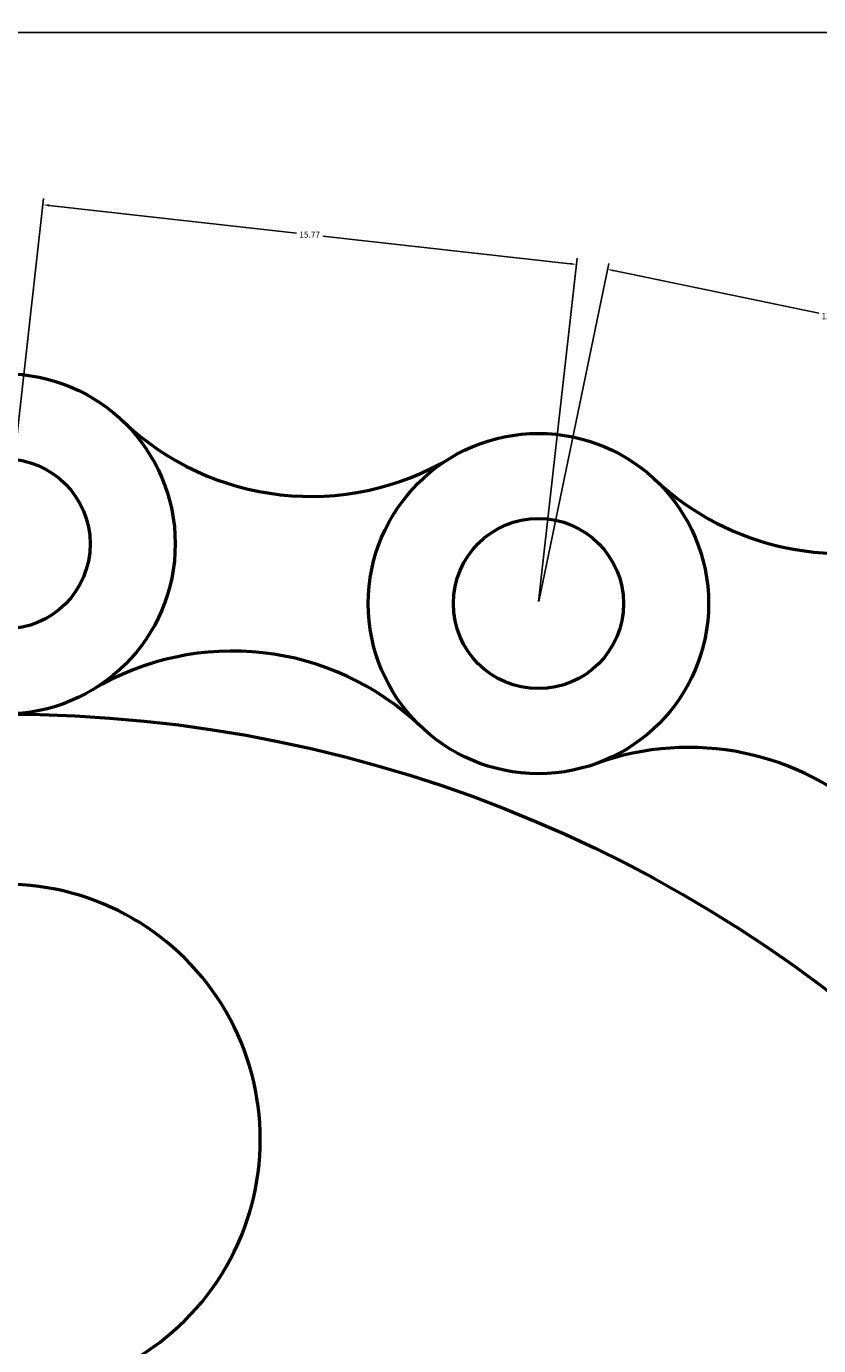
# Model space of a CAD drawing. Units: inches. Extents: x 413 to 622, y 326 to 447.
# Tile 7 of 15: x 473 to 497, y 408 to 447. Entities that reach past the tile are written whole.
import ezdxf

# ---------------------------------------------------------------- set-up
doc = ezdxf.new("R2010")
doc.units = ezdxf.units.IN
doc.header["$MEASUREMENT"] = 0
doc.layers.add('M-DIMS', color=2, linetype='Continuous', lineweight=18)
doc.layers.add('M-OUTL', color=7, linetype='Continuous', lineweight=50)
doc.styles.get("Standard").update_dxf_attribs({"font": 'arial.ttf'})
doc.dimstyles.get("Standard").update_dxf_attribs({"dimtxt": 0.18, "dimasz": 0.18, "dimexe": 0.18, "dimexo": 0.0625, "dimgap": 0.09, "dimtad": 0, "dimtih": 1, "dimtoh": 1, "dimdec": 4, "dimzin": 0, "dimdsep": 46, "dimtxsty": 'Standard', "dimcen": 0.09, "dimadec": 0, "dimazin": 0, "dimtfac": 1, "dimtdec": 4, "dimtofl": 0, "dimtmove": 0, "dimatfit": 3, "dimfxl": 1, "dimtolj": 1, "dimtzin": 0, "dimarcsym": 0})

# ---------------------------------------------------------------- blocks, each defined once
blk = doc.blocks.new('CHAIN-ROLLER-PIN')
for radius in [5, 2.5]:
    blk.add_circle((5, 5), radius)
blk = doc.blocks.new('SPROCKET-WEB-SLOT')
blk.add_arc((7.501, 21.25), 7.5, 30, 210)
blk = doc.blocks.new('CHAIN-LINK-WAIST-P15_769')
for centre, start, end in [((6.414, 14.762), 226.2787, 300.9551), ((4.115, -5.782), 46.2787, 120.9551)]:
    blk.add_arc(centre, 8, start, end)
blk = doc.blocks.new('CHAIN-LINK-WAIST-P13_603')
for centre, start, end in [((7.205, 15.87), 226.7719, 289.8627), ((2.718, -5.829), 46.7719, 109.8627)]:
    blk.add_arc(centre, 8, start, end)
blk = doc.blocks.new('*D11')
at = {"layer": 'Defpoints', "color": 0, "transparency": 16777216}
for p in [(621.66, 446.422), (621.66, 388.074), (423.314, 378.888)]:
    blk.add_point(p, dxfattribs=at)
at = {"layer": 'M-DIMS', "color": 0, "lineweight": -2, "transparency": 16777216}
for p, q in [((423.314, 378.95), (423.314, 446.602)), ((423.494, 446.422), (522.031, 446.422)), ((621.48, 446.422), (522.943, 446.422)), ((621.66, 388.137), (621.66, 446.602))]:
    blk.add_line(p, q, dxfattribs=at)
at = {"layer": 'M-DIMS', "color": 0, "transparency": 16777216}
for points in [[(423.494, 446.452), (423.494, 446.392), (423.314, 446.422)], [(621.48, 446.452), (621.48, 446.392), (621.66, 446.422)]]:
    blk.add_solid(points, dxfattribs=at)
at = {"layer": 'M-DIMS', "color": 0, "transparency": 16777216, "insert": (522.487, 446.422), "char_height": 0.18, "attachment_point": 5}
blk.add_mtext('\\A1;198.35', dxfattribs=at)
blk = doc.blocks.new('*D16')
at = {"layer": 'Defpoints', "color": 0, "transparency": 16777216}
for p in [(489.47, 439.607), (472.684, 431.392), (488.355, 429.638)]:
    blk.add_point(p, dxfattribs=at)
at = {"layer": 'M-DIMS', "color": 0, "lineweight": -2, "transparency": 16777216}
for p, q in [((472.691, 431.454), (473.819, 441.539)), ((473.978, 441.34), (481.249, 440.526)), ((489.292, 439.627), (482.02, 440.44)), ((488.362, 429.7), (489.49, 439.786))]:
    blk.add_line(p, q, dxfattribs=at)
at = {"layer": 'M-DIMS', "color": 0, "transparency": 16777216}
for points in [[(473.981, 441.37), (473.974, 441.31), (473.799, 441.36)], [(489.295, 439.656), (489.288, 439.597), (489.47, 439.607)]]:
    blk.add_solid(points, dxfattribs=at)
at = {"layer": 'M-DIMS', "color": 0, "transparency": 16777216, "insert": (481.635, 440.483), "char_height": 0.18, "attachment_point": 5}
blk.add_mtext('\\A1;15.77', dxfattribs=at)
blk = doc.blocks.new('*D17')
at = {"layer": 'Defpoints', "color": 0, "transparency": 16777216}
for p in [(503.707, 436.707), (488.355, 429.638), (501.676, 426.884)]:
    blk.add_point(p, dxfattribs=at)
at = {"layer": 'M-DIMS', "color": 0, "lineweight": -2, "transparency": 16777216}
for p, q in [((488.368, 429.7), (490.423, 439.637)), ((490.563, 439.425), (496.592, 438.178)), ((503.531, 436.743), (497.502, 437.99)), ((501.689, 426.945), (503.744, 436.883))]:
    blk.add_line(p, q, dxfattribs=at)
at = {"layer": 'M-DIMS', "color": 0, "transparency": 16777216}
for points in [[(490.569, 439.454), (490.557, 439.395), (490.386, 439.461)], [(503.537, 436.772), (503.525, 436.714), (503.707, 436.707)]]:
    blk.add_solid(points, dxfattribs=at)
at = {"layer": 'M-DIMS', "color": 0, "transparency": 16777216, "insert": (497.047, 438.084), "char_height": 0.18, "attachment_point": 5}
blk.add_mtext('\\A1;13.603', dxfattribs=at)

msp = doc.modelspace()

# ---------------------------------------------------------------- linework, layer by layer
at = {"layer": 'M-OUTL'}
msp.add_circle((472.6836, 386.3915), 40, dxfattribs=at)

# ---------------------------------------------------------------- block references
for name, p in [('CHAIN-ROLLER-PIN', (467.684, 426.392)), ('CHAIN-LINK-WAIST-P15_769', (475.255, 426.025)), ('CHAIN-ROLLER-PIN', (483.3557, 424.6388)), ('CHAIN-LINK-WAIST-P13_603', (490.054, 423.241))]:
    msp.add_blockref(name, p, dxfattribs=at)
at = {"layer": 'M-OUTL', "rotation": 239.9999999999996}
msp.add_blockref('SPROCKET-WEB-SLOT', (458.0314, 431.0122), dxfattribs=at)

# ---------------------------------------------------------------- dimensions: what is measured, and where the dimension line sits
at = {"layer": 'M-DIMS'}
dim = msp.add_linear_dim(base=(621.66, 446.422), p1=(423.3136, 378.8878), p2=(621.66, 388.0741), dimstyle='Standard', override={"dimdec": 2, "dimlfac": 1, "dimrnd": 0, "dimzin": 0, "dimdsep": 46, "dimlunit": 2}, dxfattribs=at)
dim.commit()
dim.dimension.update_dxf_attribs({"geometry": '*D11', "text_midpoint": (522.4868, 446.422)})
for base, p1, p2, angle, override, picture, middle in [((489.4705, 439.6066), (472.6836, 431.3915), (488.3553, 429.6383), 353.6169, {"dimdec": 2, "dimlfac": 1, "dimrnd": 0, "dimzin": 0, "dimdsep": 46, "dimlunit": 2}, '*D16', (481.6346, 440.4832)), ((503.7072, 436.7066), (488.3553, 429.6383), (501.6761, 426.8839), 348.31726, {"dimdec": 3, "dimlfac": 1, "dimrnd": 0, "dimzin": 0, "dimdsep": 46, "dimlunit": 2}, '*D17', (497.0468, 438.0838))]:
    dim = msp.add_linear_dim(base=base, p1=p1, p2=p2, angle=angle, dimstyle='Standard', override=override, dxfattribs=at)
    dim.commit()
    dim.dimension.update_dxf_attribs({"geometry": picture, "text_midpoint": middle})

doc.saveas('drawing.dxf')
